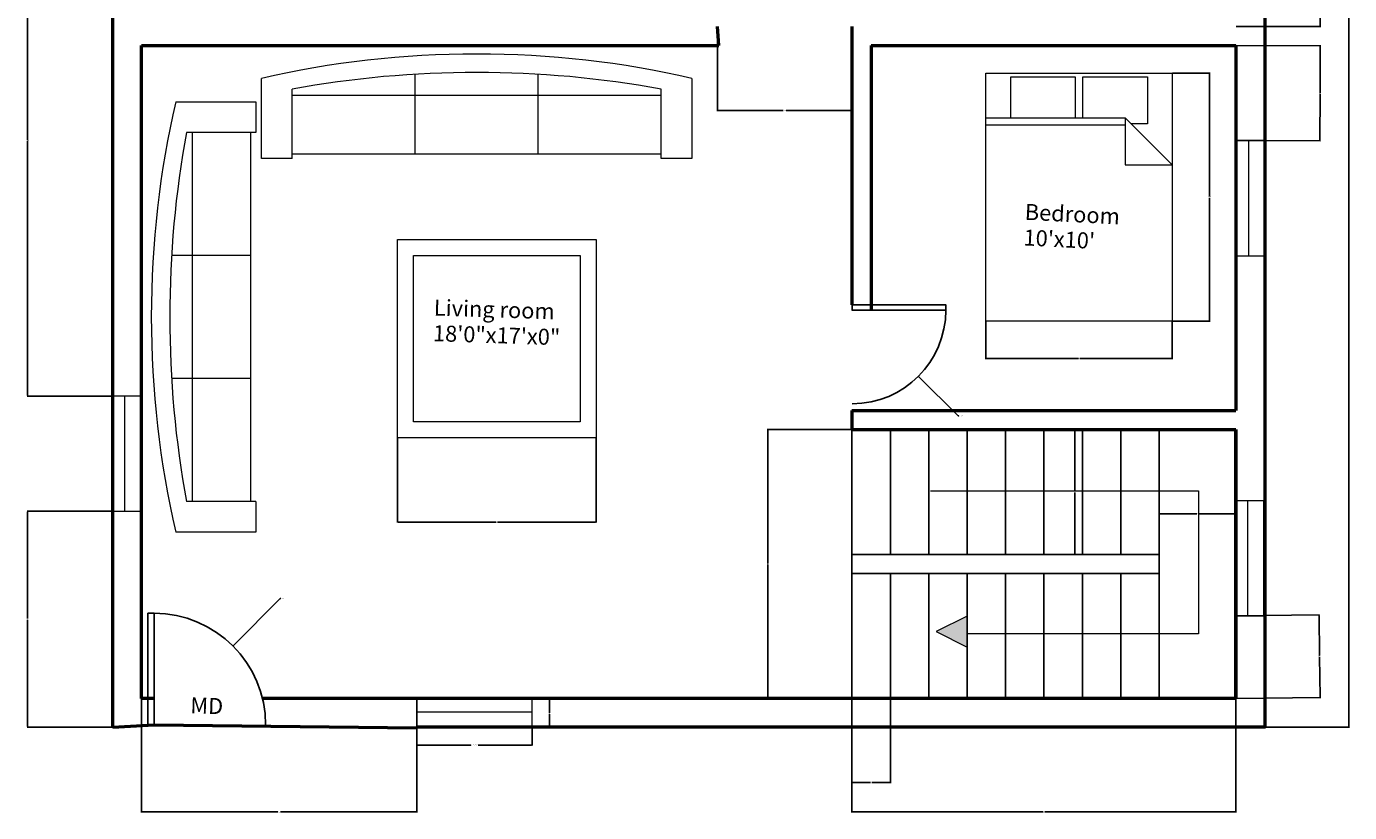
# Model space of a CAD drawing. Units: feet. Extents: x 2128 to 3163, y 1733 to 2266.
# Tile 2 of 3: x 2750 to 3163, y 1733 to 1979. Entities that reach past the tile are written whole.
import ezdxf

# ---------------------------------------------------------------- set-up
doc = ezdxf.new("R2010")
doc.units = ezdxf.units.FT
for name, color, linetype, lineweight in [('A-ANNO-DIMS', 2, 'Continuous', 18), ('A-ANNO-SYMB', 2, 'Continuous', 18), ('A-ANNO-TEXT', 7, 'Continuous', 18), ('A-AREA-IDEN', 7, 'Continuous', 18), ('A-DOOR', 3, 'Continuous', 25), ('A-FLOR-STRS', 7, 'Continuous', 25), ('A-FURN', 8, 'Continuous', 18), ('A-GLAZ', 4, 'Continuous', 18), ('A-WALL', 7, 'Continuous', 50)]:
    doc.layers.add(name, color=color, linetype=linetype, lineweight=lineweight)
doc.styles.get("Standard").update_dxf_attribs({"font": 'arial.ttf'})
doc.dimstyles.get("Standard").update_dxf_attribs({"dimtxt": 0.18, "dimasz": 0.18, "dimexe": 0.18, "dimexo": 0.0625, "dimgap": 0.09, "dimtad": 0, "dimtih": 1, "dimtoh": 1, "dimdec": 4, "dimzin": 0, "dimdsep": 46, "dimtxsty": 'Standard', "dimcen": 0.09, "dimadec": 0, "dimazin": 0, "dimtfac": 1, "dimtdec": 4, "dimtofl": 0, "dimtmove": 0, "dimatfit": 3, "dimfxl": 1, "dimtolj": 1, "dimtzin": 0, "dimarcsym": 0})

# ---------------------------------------------------------------- blocks, each defined once
blk = doc.blocks.new('Bed - Queen')
for p, q in [((0, -80.00003), (0, 0)), ((0, 0), (59.99999, 0)), ((59.99999, 0), (59.99999, -80.00003)), ((7.99999, -1.2), (28.79998, -1.2)), ((7.99999, -14.4), (7.99999, -1.2)), ((28.79998, -1.2), (28.79998, -14.4)), ((31.19999, -1.2), (51.99999, -1.2)), ((31.19999, -14.4), (31.19999, -1.2)), ((51.99999, -1.2), (51.99999, -16.4)), ((0, -14.4), (44.8, -14.4)), ((44.8, -16.8), (0, -16.8)), ((59.99999, -29.6), (44.8, -14.4)), ((44.8, -14.4), (44.8, -29.6)), ((51.99999, -16.4), (46.79936, -16.4)), ((44.8, -29.6), (59.99999, -29.6)), ((59.99999, -80.00003), (0, -80.00003))]:
    blk.add_line(p, q)
blk = doc.blocks.new('Sofa - Roundback 7 ft.')
for p, q in [((-12.00002, -32.4421), (-12.00003, -6.5971)), ((11.99997, -32.4421), (11.99998, -6.5971)), ((-36.000027, -34), (-36.000027, -11.4696)), ((35.99998, -34), (35.99998, -11.4696)), ((-35.999844, -13.3819), (35.9998, -13.3819)), ((-36.000027, -32.4421), (35.99998, -32.4421))]:
    blk.add_line(p, q)
for points in [[(-36.000027, -34), (-42.000027, -34), (-42.000027, -8)], [(41.99998, -8), (41.99998, -34), (35.99998, -34)]]:
    blk.add_lwpolyline(points)
for centre, radius, start, end in [((0, -114.25), 114.25, 68.43141, 111.5686), ((-0.00001, -127.1968), 121.1968, 72.72033, 107.2797)]:
    blk.add_arc(centre, radius, start, end)
blk = doc.blocks.new('DOOR-INTERIOR-SWING')
blk.add_lwpolyline([(1.63, 0), (0, 0), (0, 29.25), (1.63, 29.25)], close=True)
blk.add_arc((1.63, 0), 29.25, 0, 90)
blk = doc.blocks.new('WIN-SINGLE-36')
blk.add_line((0.01, 4.96), (35.9, 4.96))
blk.add_lwpolyline([(36, 9), (0, 9), (0, 0), (36, 0)], close=True)
blk = doc.blocks.new('*D9')
at = {"layer": 'A-ANNO-DIMS', "color": 0, "lineweight": -2, "transparency": 16777216}
for p, q in [((2871.76, 1759.28), (2871.76, 1753.77)), ((2907.76, 1759.28), (2907.76, 1753.77)), ((2871.94, 1753.95), (2888.65, 1753.95)), ((2907.58, 1753.95), (2890.88, 1753.95))]:
    blk.add_line(p, q, dxfattribs=at)
at = {"layer": 'A-ANNO-DIMS', "color": 0, "transparency": 16777216}
for points in [[(2871.94, 1753.98), (2871.94, 1753.92), (2871.76, 1753.95)], [(2907.58, 1753.98), (2907.58, 1753.92), (2907.76, 1753.95)]]:
    blk.add_solid(points, dxfattribs=at)
at = {"layer": 'Defpoints', "color": 0, "transparency": 16777216}
for p in [(2871.76, 1759.35), (2907.76, 1759.35), (2907.76, 1753.95)]:
    blk.add_point(p, dxfattribs=at)
at = {"layer": 'A-ANNO-DIMS', "color": 0, "transparency": 16777216, "insert": (2889.76, 1753.95), "char_height": 0.18, "attachment_point": 5}
blk.add_mtext('\\A1;WINDOW 36 TYP.', dxfattribs=at)
blk = doc.blocks.new('*D10')
at = {"layer": 'A-ANNO-DIMS', "color": 0, "lineweight": -2, "transparency": 16777216}
for p, q in [((2907.83, 1768.35), (2913.34, 1768.35)), ((2913.16, 1768.17), (2913.16, 1764.03)), ((2913.16, 1759.53), (2913.16, 1763.66)), ((2907.83, 1759.35), (2913.34, 1759.35))]:
    blk.add_line(p, q, dxfattribs=at)
at = {"layer": 'A-ANNO-DIMS', "color": 0, "transparency": 16777216}
for points in [[(2913.13, 1768.17), (2913.19, 1768.17), (2913.16, 1768.35)], [(2913.13, 1759.53), (2913.19, 1759.53), (2913.16, 1759.35)]]:
    blk.add_solid(points, dxfattribs=at)
at = {"layer": 'Defpoints', "color": 0, "transparency": 16777216}
for p in [(2907.76, 1768.35), (2913.16, 1768.35), (2907.76, 1759.35)]:
    blk.add_point(p, dxfattribs=at)
at = {"layer": 'A-ANNO-DIMS', "color": 0, "transparency": 16777216, "insert": (2913.16, 1763.85), "char_height": 0.18, "attachment_point": 5}
blk.add_mtext('\\A1;9 TYP.', dxfattribs=at)
blk = doc.blocks.new('*D17')
at = {"layer": 'A-ANNO-DIMS', "color": 0, "lineweight": -2, "transparency": 16777216}
for p, q in [((3107.89, 1963.99), (3119.64, 1963.99)), ((3119.46, 1963.81), (3119.46, 1925.39)), ((3119.46, 1886.61), (3119.46, 1925.03)), ((3107.89, 1886.43), (3119.64, 1886.43))]:
    blk.add_line(p, q, dxfattribs=at)
at = {"layer": 'A-ANNO-DIMS', "color": 0, "transparency": 16777216}
for points in [[(3119.43, 1963.81), (3119.49, 1963.81), (3119.46, 1963.99)], [(3119.43, 1886.61), (3119.49, 1886.61), (3119.46, 1886.43)]]:
    blk.add_solid(points, dxfattribs=at)
at = {"layer": 'Defpoints', "color": 0, "transparency": 16777216}
for p in [(3107.82, 1963.99), (3119.46, 1963.99), (3107.82, 1886.43)]:
    blk.add_point(p, dxfattribs=at)
at = {"layer": 'A-ANNO-DIMS', "color": 0, "transparency": 16777216, "insert": (3119.46, 1925.21), "char_height": 0.18, "attachment_point": 5}
blk.add_mtext('\\A1;BED 78', dxfattribs=at)
blk = doc.blocks.new('*D18')
at = {"layer": 'A-ANNO-DIMS', "color": 0, "lineweight": -2, "transparency": 16777216}
for p, q in [((3049.6, 1886.36), (3049.6, 1874.61)), ((3107.82, 1886.36), (3107.82, 1874.61)), ((3049.78, 1874.79), (3078.49, 1874.79)), ((3107.64, 1874.79), (3078.93, 1874.79))]:
    blk.add_line(p, q, dxfattribs=at)
at = {"layer": 'A-ANNO-DIMS', "color": 0, "transparency": 16777216}
for points in [[(3049.78, 1874.82), (3049.78, 1874.76), (3049.6, 1874.79)], [(3107.64, 1874.82), (3107.64, 1874.76), (3107.82, 1874.79)]]:
    blk.add_solid(points, dxfattribs=at)
at = {"layer": 'Defpoints', "color": 0, "transparency": 16777216}
for p in [(3049.6, 1886.43), (3107.82, 1886.43), (3107.82, 1874.79)]:
    blk.add_point(p, dxfattribs=at)
at = {"layer": 'A-ANNO-DIMS', "color": 0, "transparency": 16777216, "insert": (3078.71, 1874.79), "char_height": 0.18, "attachment_point": 5}
blk.add_mtext('\\A1;58', dxfattribs=at)
blk = doc.blocks.new('*D26')
at = {"layer": 'A-ANNO-DIMS', "color": 0, "lineweight": -2, "transparency": 16777216}
for p, q in [((3136.8, 2239.55), (3163.22, 2239.55)), ((3163.04, 2239.37), (3163.04, 1999.73)), ((3163.04, 1759.73), (3163.04, 1999.36)), ((3136.8, 1759.55), (3163.22, 1759.55))]:
    blk.add_line(p, q, dxfattribs=at)
at = {"layer": 'A-ANNO-DIMS', "color": 0, "transparency": 16777216}
for points in [[(3163.01, 2239.37), (3163.07, 2239.37), (3163.04, 2239.55)], [(3163.01, 1759.73), (3163.07, 1759.73), (3163.04, 1759.55)]]:
    blk.add_solid(points, dxfattribs=at)
at = {"layer": 'Defpoints', "color": 0, "transparency": 16777216}
for p in [(3136.74, 2239.55), (3136.74, 1759.55), (3163.04, 1759.55)]:
    blk.add_point(p, dxfattribs=at)
at = {"layer": 'A-ANNO-DIMS', "color": 0, "transparency": 16777216, "insert": (3163.04, 1999.55), "char_height": 0.18, "attachment_point": 5}
blk.add_mtext('\\A1;480', dxfattribs=at)
blk = doc.blocks.new('*D29')
at = {"layer": 'A-ANNO-DIMS', "color": 0, "lineweight": -2, "transparency": 16777216}
for p, q in [((2785.74, 1768.48), (2785.74, 1732.87)), ((2871.76, 1768.28), (2871.76, 1732.87)), ((2785.92, 1733.05), (2828.36, 1733.05)), ((2871.58, 1733.05), (2829.14, 1733.05))]:
    blk.add_line(p, q, dxfattribs=at)
at = {"layer": 'A-ANNO-DIMS', "color": 0, "transparency": 16777216}
for points in [[(2785.92, 1733.08), (2785.92, 1733.02), (2785.74, 1733.05)], [(2871.58, 1733.08), (2871.58, 1733.02), (2871.76, 1733.05)]]:
    blk.add_solid(points, dxfattribs=at)
at = {"layer": 'Defpoints', "color": 0, "transparency": 16777216}
for p in [(2785.74, 1768.55), (2871.76, 1768.35), (2871.76, 1733.05)]:
    blk.add_point(p, dxfattribs=at)
at = {"layer": 'A-ANNO-DIMS', "color": 0, "transparency": 16777216, "insert": (2828.75, 1733.05), "char_height": 0.18, "attachment_point": 5}
blk.add_mtext('\\A1;86.03', dxfattribs=at)
blk = doc.blocks.new('*D31')
at = {"layer": 'A-ANNO-DIMS', "color": 0, "lineweight": -2, "transparency": 16777216}
for p, q in [((3127.79, 2004.71), (3154.21, 2004.71)), ((3154.03, 2004.53), (3154.03, 1991.81)), ((3154.04, 1978.73), (3154.03, 1991.45)), ((3127.8, 1978.55), (3154.22, 1978.55))]:
    blk.add_line(p, q, dxfattribs=at)
at = {"layer": 'A-ANNO-DIMS', "color": 0, "transparency": 16777216}
for points in [[(3154.06, 2004.53), (3154, 2004.53), (3154.03, 2004.71)], [(3154.07, 1978.73), (3154.01, 1978.73), (3154.04, 1978.55)]]:
    blk.add_solid(points, dxfattribs=at)
at = {"layer": 'Defpoints', "color": 0, "transparency": 16777216}
for p in [(3127.73, 2004.71), (3127.74, 1978.55), (3154.04, 1978.55)]:
    blk.add_point(p, dxfattribs=at)
at = {"layer": 'A-ANNO-DIMS', "color": 0, "transparency": 16777216, "insert": (3154.03, 1991.63), "char_height": 0.18, "attachment_point": 5}
blk.add_mtext('\\A1;26.16', dxfattribs=at)
blk = doc.blocks.new('*D33')
at = {"layer": 'A-ANNO-DIMS', "color": 0, "lineweight": -2, "transparency": 16777216}
for p, q in [((3127.8, 1972.55), (3154.22, 1972.49)), ((3154.04, 1972.32), (3154.01, 1957.84)), ((3153.98, 1943), (3154.01, 1957.48)), ((3127.74, 1942.87), (3154.16, 1942.82))]:
    blk.add_line(p, q, dxfattribs=at)
at = {"layer": 'A-ANNO-DIMS', "color": 0, "transparency": 16777216}
for points in [[(3154.01, 1972.32), (3154.07, 1972.32), (3154.04, 1972.5)], [(3153.95, 1943), (3154.01, 1943), (3153.98, 1942.82)]]:
    blk.add_solid(points, dxfattribs=at)
at = {"layer": 'Defpoints', "color": 0, "transparency": 16777216}
for p in [(3127.74, 1972.55), (3127.68, 1942.87), (3153.98, 1942.82)]:
    blk.add_point(p, dxfattribs=at)
at = {"layer": 'A-ANNO-DIMS', "color": 0, "transparency": 16777216, "insert": (3154.01, 1957.66), "char_height": 0.18, "attachment_point": 5}
blk.add_mtext('\\A1;29.67', dxfattribs=at)
blk = doc.blocks.new('*D34')
at = {"layer": 'A-ANNO-DIMS', "color": 0, "lineweight": -2, "transparency": 16777216}
for p, q in [((3127.48, 1794.33), (3153.9, 1794.66)), ((3153.72, 1794.48), (3153.87, 1781.94)), ((3154.03, 1769.05), (3153.88, 1781.58)), ((3127.8, 1768.55), (3154.22, 1768.87))]:
    blk.add_line(p, q, dxfattribs=at)
at = {"layer": 'A-ANNO-DIMS', "color": 0, "transparency": 16777216}
for points in [[(3153.75, 1794.48), (3153.69, 1794.48), (3153.72, 1794.66)], [(3154.06, 1769.05), (3154, 1769.05), (3154.04, 1768.87)]]:
    blk.add_solid(points, dxfattribs=at)
at = {"layer": 'Defpoints', "color": 0, "transparency": 16777216}
for p in [(3127.42, 1794.33), (3127.74, 1768.55), (3154.04, 1768.87)]:
    blk.add_point(p, dxfattribs=at)
at = {"layer": 'A-ANNO-DIMS', "color": 0, "transparency": 16777216, "insert": (3153.88, 1781.76), "char_height": 0.18, "attachment_point": 5}
blk.add_mtext('\\A1;25.79', dxfattribs=at)
blk = doc.blocks.new('*D35')
at = {"layer": 'A-ANNO-DIMS', "color": 0, "lineweight": -2, "transparency": 16777216}
for p, q in [((3007.67, 1852.55), (2981.26, 1852.55)), ((2981.44, 1852.37), (2981.44, 1810.73)), ((2981.44, 1768.73), (2981.44, 1810.36)), ((3007.67, 1768.55), (2981.26, 1768.55))]:
    blk.add_line(p, q, dxfattribs=at)
at = {"layer": 'A-ANNO-DIMS', "color": 0, "transparency": 16777216}
for points in [[(2981.41, 1852.37), (2981.47, 1852.37), (2981.44, 1852.55)], [(2981.41, 1768.73), (2981.47, 1768.73), (2981.44, 1768.55)]]:
    blk.add_solid(points, dxfattribs=at)
at = {"layer": 'Defpoints', "color": 0, "transparency": 16777216}
for p in [(2981.44, 1852.55), (3007.74, 1852.55), (3007.74, 1768.55)]:
    blk.add_point(p, dxfattribs=at)
at = {"layer": 'A-ANNO-DIMS', "color": 0, "transparency": 16777216, "insert": (2981.44, 1810.55), "char_height": 0.18, "attachment_point": 5}
blk.add_mtext('\\A1;84', dxfattribs=at)
blk = doc.blocks.new('*D36')
at = {"layer": 'A-ANNO-DIMS', "color": 0, "lineweight": -2, "transparency": 16777216}
for p, q in [((3007.74, 1768.48), (3007.74, 1732.87)), ((3127.74, 1768.48), (3127.74, 1732.87)), ((3007.92, 1733.05), (3067.46, 1733.05)), ((3127.56, 1733.05), (3068.02, 1733.05))]:
    blk.add_line(p, q, dxfattribs=at)
at = {"layer": 'A-ANNO-DIMS', "color": 0, "transparency": 16777216}
for points in [[(3007.92, 1733.08), (3007.92, 1733.02), (3007.74, 1733.05)], [(3127.56, 1733.08), (3127.56, 1733.02), (3127.74, 1733.05)]]:
    blk.add_solid(points, dxfattribs=at)
at = {"layer": 'Defpoints', "color": 0, "transparency": 16777216}
for p in [(3007.74, 1768.55), (3127.74, 1768.55), (3127.74, 1733.05)]:
    blk.add_point(p, dxfattribs=at)
at = {"layer": 'A-ANNO-DIMS', "color": 0, "transparency": 16777216, "insert": (3067.74, 1733.05), "char_height": 0.18, "attachment_point": 5}
blk.add_mtext('\\A1;120', dxfattribs=at)
blk = doc.blocks.new('*D37')
at = {"layer": 'A-ANNO-DIMS', "color": 0, "lineweight": -2, "transparency": 16777216}
for p, q in [((3007.74, 1768.48), (3007.74, 1742.07)), ((3019.74, 1768.48), (3019.74, 1742.07)), ((3007.92, 1742.25), (3013.53, 1742.25)), ((3019.56, 1742.25), (3013.95, 1742.25))]:
    blk.add_line(p, q, dxfattribs=at)
at = {"layer": 'A-ANNO-DIMS', "color": 0, "transparency": 16777216}
for points in [[(3007.92, 1742.28), (3007.92, 1742.22), (3007.74, 1742.25)], [(3019.56, 1742.28), (3019.56, 1742.22), (3019.74, 1742.25)]]:
    blk.add_solid(points, dxfattribs=at)
at = {"layer": 'Defpoints', "color": 0, "transparency": 16777216}
for p in [(3007.74, 1768.55), (3019.74, 1768.55), (3007.74, 1742.25)]:
    blk.add_point(p, dxfattribs=at)
at = {"layer": 'A-ANNO-DIMS', "color": 0, "transparency": 16777216, "insert": (3013.74, 1742.25), "char_height": 0.18, "attachment_point": 5}
blk.add_mtext('\\A1;12', dxfattribs=at)
blk = doc.blocks.new('*D38')
at = {"layer": 'A-ANNO-DIMS', "color": 0, "lineweight": -2, "transparency": 16777216}
for p, q in [((3103.74, 1852.48), (3103.74, 1826.07)), ((3127.74, 1852.48), (3127.74, 1826.07)), ((3103.92, 1826.25), (3115.52, 1826.25)), ((3127.56, 1826.25), (3115.96, 1826.25))]:
    blk.add_line(p, q, dxfattribs=at)
at = {"layer": 'A-ANNO-DIMS', "color": 0, "transparency": 16777216}
for points in [[(3103.92, 1826.28), (3103.92, 1826.22), (3103.74, 1826.25)], [(3127.56, 1826.28), (3127.56, 1826.22), (3127.74, 1826.25)]]:
    blk.add_solid(points, dxfattribs=at)
at = {"layer": 'Defpoints', "color": 0, "transparency": 16777216}
for p in [(3103.74, 1852.55), (3127.74, 1852.55), (3103.74, 1826.25)]:
    blk.add_point(p, dxfattribs=at)
at = {"layer": 'A-ANNO-DIMS', "color": 0, "transparency": 16777216, "insert": (3115.74, 1826.25), "char_height": 0.18, "attachment_point": 5}
blk.add_mtext('\\A1;24', dxfattribs=at)
blk = doc.blocks.new('*D39')
at = {"layer": 'A-ANNO-DIMS', "color": 0, "lineweight": -2, "transparency": 16777216}
for p, q in [((3103.67, 1852.55), (3077.26, 1852.55)), ((3077.44, 1852.37), (3077.44, 1833.23)), ((3077.44, 1813.73), (3077.44, 1832.86)), ((3103.67, 1813.55), (3077.26, 1813.55))]:
    blk.add_line(p, q, dxfattribs=at)
at = {"layer": 'A-ANNO-DIMS', "color": 0, "transparency": 16777216}
for points in [[(3077.41, 1852.37), (3077.47, 1852.37), (3077.44, 1852.55)], [(3077.41, 1813.73), (3077.47, 1813.73), (3077.44, 1813.55)]]:
    blk.add_solid(points, dxfattribs=at)
at = {"layer": 'Defpoints', "color": 0, "transparency": 16777216}
for p in [(3077.44, 1852.55), (3103.74, 1852.55), (3103.74, 1813.55)]:
    blk.add_point(p, dxfattribs=at)
at = {"layer": 'A-ANNO-DIMS', "color": 0, "transparency": 16777216, "insert": (3077.44, 1833.05), "char_height": 0.18, "attachment_point": 5}
blk.add_mtext('\\A1;39', dxfattribs=at)
blk = doc.blocks.new('*D40')
at = {"layer": 'A-ANNO-DIMS', "color": 0, "lineweight": -2, "transparency": 16777216}
for p, q in [((2776.42, 1827.05), (2749.94, 1827.05)), ((2750.12, 1826.87), (2750.12, 1793.48)), ((2750.12, 1759.73), (2750.12, 1793.11)), ((2776.67, 1759.55), (2749.94, 1759.55))]:
    blk.add_line(p, q, dxfattribs=at)
at = {"layer": 'A-ANNO-DIMS', "color": 0, "transparency": 16777216}
for points in [[(2750.09, 1826.87), (2750.15, 1826.87), (2750.12, 1827.05)], [(2750.09, 1759.73), (2750.15, 1759.73), (2750.12, 1759.55)]]:
    blk.add_solid(points, dxfattribs=at)
at = {"layer": 'Defpoints', "color": 0, "transparency": 16777216}
for p in [(2750.12, 1827.05), (2776.49, 1827.05), (2776.74, 1759.55)]:
    blk.add_point(p, dxfattribs=at)
at = {"layer": 'A-ANNO-DIMS', "color": 0, "transparency": 16777216, "insert": (2750.12, 1793.3), "char_height": 0.18, "attachment_point": 5}
blk.add_mtext('\\A1;67.5', dxfattribs=at)
blk = doc.blocks.new('*D41')
at = {"layer": 'A-ANNO-DIMS', "color": 0, "lineweight": -2, "transparency": 16777216}
for p, q in [((2776.5, 2022.82), (2749.94, 2022.82)), ((2750.12, 2022.64), (2750.12, 1943.11)), ((2750.12, 1863.23), (2750.12, 1942.75)), ((2776.42, 1863.05), (2749.94, 1863.05))]:
    blk.add_line(p, q, dxfattribs=at)
at = {"layer": 'A-ANNO-DIMS', "color": 0, "transparency": 16777216}
for points in [[(2750.09, 2022.64), (2750.15, 2022.64), (2750.12, 2022.82)], [(2750.09, 1863.23), (2750.15, 1863.23), (2750.12, 1863.05)]]:
    blk.add_solid(points, dxfattribs=at)
at = {"layer": 'Defpoints', "color": 0, "transparency": 16777216}
for p in [(2750.12, 2022.82), (2776.56, 2022.82), (2776.49, 1863.05)]:
    blk.add_point(p, dxfattribs=at)
at = {"layer": 'A-ANNO-DIMS', "color": 0, "transparency": 16777216, "insert": (2750.12, 1942.93), "char_height": 0.18, "attachment_point": 5}
blk.add_mtext('\\A1;159.77', dxfattribs=at)
blk = doc.blocks.new('*D45')
at = {"layer": 'A-ANNO-DIMS', "color": 0, "lineweight": -2, "transparency": 16777216}
for p, q in [((2865.75, 1849.89), (2865.75, 1823.47)), ((2927.75, 1849.89), (2927.75, 1823.47)), ((2865.93, 1823.65), (2896.53, 1823.65)), ((2927.57, 1823.65), (2896.97, 1823.65))]:
    blk.add_line(p, q, dxfattribs=at)
at = {"layer": 'A-ANNO-DIMS', "color": 0, "transparency": 16777216}
for points in [[(2865.93, 1823.68), (2865.93, 1823.62), (2865.75, 1823.65)], [(2927.57, 1823.68), (2927.57, 1823.62), (2927.75, 1823.65)]]:
    blk.add_solid(points, dxfattribs=at)
at = {"layer": 'Defpoints', "color": 0, "transparency": 16777216}
for p in [(2865.75, 1849.95), (2927.75, 1849.95), (2865.75, 1823.65)]:
    blk.add_point(p, dxfattribs=at)
at = {"layer": 'A-ANNO-DIMS', "color": 0, "transparency": 16777216, "insert": (2896.75, 1823.65), "char_height": 0.18, "attachment_point": 5}
blk.add_mtext('\\A1;62', dxfattribs=at)
blk = doc.blocks.new('*D49')
at = {"layer": 'A-ANNO-DIMS', "color": 0, "lineweight": -2, "transparency": 16777216}
for p, q in [((2965.74, 1978.48), (2965.74, 1952.07)), ((3007.74, 1978.48), (3007.74, 1952.07)), ((2965.92, 1952.25), (2986.27, 1952.25)), ((3007.56, 1952.25), (2987.21, 1952.25))]:
    blk.add_line(p, q, dxfattribs=at)
at = {"layer": 'A-ANNO-DIMS', "color": 0, "transparency": 16777216}
for points in [[(2965.92, 1952.28), (2965.92, 1952.22), (2965.74, 1952.25)], [(3007.56, 1952.28), (3007.56, 1952.22), (3007.74, 1952.25)]]:
    blk.add_solid(points, dxfattribs=at)
at = {"layer": 'Defpoints', "color": 0, "transparency": 16777216}
for p in [(2965.74, 1978.55), (3007.74, 1978.55), (2965.74, 1952.25)]:
    blk.add_point(p, dxfattribs=at)
at = {"layer": 'A-ANNO-DIMS', "color": 0, "transparency": 16777216, "insert": (2986.74, 1952.25), "char_height": 0.18, "attachment_point": 5}
blk.add_mtext('\\A1;41.996', dxfattribs=at)
blk = doc.blocks.new('*D52')
at = {"layer": 'A-ANNO-DIMS', "color": 0, "lineweight": -2, "transparency": 16777216}
for p, q in [((2829.07, 1799.71), (2814.41, 1785.05)), ((2829.25, 1799.71), (2829.07, 1799.71)), ((2789.55, 1760.28), (2789.73, 1760.28)), ((2789.64, 1760.19), (2789.64, 1760.37))]:
    blk.add_line(p, q, dxfattribs=at)
at = {"layer": 'A-ANNO-DIMS', "color": 0, "transparency": 16777216}
blk.add_solid([(2814.39, 1785.08), (2814.43, 1785.03), (2814.28, 1784.93)], dxfattribs=at)
at = {"layer": 'Defpoints', "color": 0, "transparency": 16777216}
for p in [(2814.28, 1784.93), (2789.64, 1760.28)]:
    blk.add_point(p, dxfattribs=at)
at = {"layer": 'A-ANNO-DIMS', "color": 0, "transparency": 16777216, "insert": (2829.8, 1799.71), "char_height": 0.18, "attachment_point": 5}
blk.add_mtext('\\A1;R34.854', dxfattribs=at)
blk = doc.blocks.new('*D53')
at = {"layer": 'A-ANNO-DIMS', "color": 0, "lineweight": -2, "transparency": 16777216}
for p, q in [((3007.75, 1889.9), (3007.93, 1889.9)), ((3007.84, 1889.81), (3007.84, 1889.99)), ((3040.93, 1856.8), (3028.65, 1869.08)), ((3041.11, 1856.8), (3040.93, 1856.8))]:
    blk.add_line(p, q, dxfattribs=at)
at = {"layer": 'A-ANNO-DIMS', "color": 0, "transparency": 16777216}
blk.add_solid([(3028.67, 1869.11), (3028.63, 1869.06), (3028.52, 1869.21)], dxfattribs=at)
at = {"layer": 'Defpoints', "color": 0, "transparency": 16777216}
for p in [(3007.84, 1889.9), (3028.52, 1869.21)]:
    blk.add_point(p, dxfattribs=at)
at = {"layer": 'A-ANNO-DIMS', "color": 0, "transparency": 16777216, "insert": (3041.86, 1856.8), "char_height": 0.18, "attachment_point": 5}
blk.add_mtext('\\A1;3X R29.255', dxfattribs=at)

msp = doc.modelspace()

# ---------------------------------------------------------------- hatches: boundary and pattern name
at = {"layer": 'A-ANNO-SYMB'}
h = msp.add_hatch(color=256, dxfattribs=at)
h.dxf.hatch_style = 1
h.paths.add_polyline_path([(3043.737, 1794.2137), (3034.0015, 1789.4301), (3043.737, 1784.5668)])

# ---------------------------------------------------------------- linework, layer by layer
for p, q in [((3032.3072, 1833.4364), (3116.0327, 1833.4364)), ((3116.0327, 1833.4364), (3116.0327, 1788.7203)), ((3043.737, 1794.2137), (3034.0015, 1789.4301)), ((3034.0015, 1789.4301), (3043.7249, 1784.5728)), ((3116.0327, 1788.7203), (3043.8822, 1788.7203))]:
    msp.add_line(p, q, dxfattribs=at)
at = {"layer": 'A-DOOR'}
msp.add_lwpolyline([(2789.6368, 1760.281), (2787.7005, 1760.281), (2787.7005, 1795.1352), (2789.6368, 1795.1352)], close=True, dxfattribs=at)
msp.add_arc((2789.6368, 1760.281), 34.8542, 0, 90, dxfattribs=at)
at = {"layer": 'A-FLOR-STRS'}
for p, q in [((3007.737, 1768.546), (3007.737, 1852.546)), ((3019.737, 1813.546), (3019.737, 1852.546)), ((3031.737, 1813.546), (3031.737, 1852.546)), ((3043.737, 1813.546), (3043.737, 1852.546)), ((3055.737, 1813.546), (3055.737, 1852.546)), ((3067.737, 1813.546), (3067.737, 1852.546)), ((3079.737, 1813.546), (3079.737, 1852.546)), ((3091.737, 1813.546), (3091.737, 1852.546)), ((3103.737, 1768.546), (3103.737, 1852.546)), ((3007.737, 1813.546), (3103.737, 1813.546)), ((3007.737, 1807.546), (3103.737, 1807.546)), ((3019.737, 1768.546), (3019.737, 1807.546)), ((3031.737, 1768.546), (3031.737, 1807.546)), ((3043.737, 1768.546), (3043.737, 1807.546)), ((3055.737, 1768.546), (3055.737, 1807.546)), ((3067.737, 1768.546), (3067.737, 1807.546)), ((3079.737, 1768.546), (3079.737, 1807.546)), ((3091.737, 1768.546), (3091.737, 1807.546))]:
    msp.add_line(p, q, dxfattribs=at)
at = {"layer": 'A-FURN'}
for points in [[(2865.7512, 1911.9544), (2927.7512, 1911.9544), (2927.7512, 1849.9544), (2865.7512, 1849.9544)], [(2870.7512, 1906.9544), (2922.7512, 1906.9544), (2922.7512, 1854.9544), (2870.7512, 1854.9544)]]:
    msp.add_lwpolyline(points, close=True, dxfattribs=at)
at = {"layer": 'A-WALL'}
for p, q in [((2966.0879, 1972.546), (2965.7414, 1978.546)), ((3007.737, 1978.546), (3007.737, 1891.5229)), ((2785.737, 1768.546), (2785.737, 1972.546)), ((2785.737, 1972.546), (2953.737, 1972.546)), ((2953.737, 1972.546), (2966.0879, 1972.546)), ((3013.737, 1972.546), (3013.737, 1889.8976)), ((3013.737, 1972.546), (3127.737, 1972.546)), ((3127.737, 1972.546), (3127.737, 1858.546)), ((3007.8364, 1891.5229), (3007.737, 1891.5229)), ((3007.737, 1858.546), (3127.737, 1858.546)), ((3007.737, 1858.546), (3007.737, 1852.546)), ((3007.737, 1852.546), (3127.737, 1852.546)), ((3127.737, 1768.546), (3127.737, 1852.546)), ((3127.737, 1852.546), (3127.737, 1768.546)), ((2789.6368, 1768.546), (2785.737, 1768.546)), ((3127.737, 1768.546), (2823.4969, 1768.546)), ((2776.737, 1759.546), (2789.6368, 1760.281)), ((2789.6368, 1760.281), (2871.7638, 1759.3457))]:
    msp.add_line(p, q, dxfattribs=at)
msp.add_lwpolyline([(2776.737, 1759.546), (2776.737, 2239.546), (3136.737, 2239.546), (3136.737, 1759.546), (2871.7638, 1759.546)], dxfattribs=at)

# ---------------------------------------------------------------- block references
at = {"layer": 'A-DOOR', "rotation": 270.0000000000013}
msp.add_blockref('DOOR-INTERIOR-SWING', (3007.8364, 1891.5232), dxfattribs=at)
at = {"layer": 'A-FURN', "xscale": 1.601553536944322, "yscale": 0.9600654288777931, "zscale": 1.601553536944322}
msp.add_blockref('Sofa - Roundback 7 ft.', (2890.4559, 1969.9316), dxfattribs=at)
at = {"layer": 'A-FURN'}
for name, p, xscale, yscale, zscale, rotation in [('Bed - Queen', (3049.5954, 1963.9936), -0.9704664129428286, -0.9695930824229791, 0.9704664129428286, 180), ('Sofa - Roundback 7 ft.', (2788.7678, 1887.7649), 1.601553536944322, 0.9600654288777931, 1.601553536944322, 90)]:
    msp.add_blockref(name, p, dxfattribs=dict(at, xscale=xscale, yscale=yscale, zscale=zscale, rotation=rotation))
at = {"layer": 'A-GLAZ'}
for p, rotation in [((3136.6792, 1906.8748), 89.99999999999808), ((2785.487, 1827.0466), 90.0000000000003), ((3136.4194, 1794.3335), 89.99999999999523)]:
    msp.add_blockref('WIN-SINGLE-36', p, dxfattribs=dict(at, rotation=rotation))
msp.add_blockref('WIN-SINGLE-36', (2871.7641, 1759.3461), dxfattribs=at)

# ---------------------------------------------------------------- texts
at = {"layer": 'A-ANNO-TEXT'}
msp.add_text('MD', height=5, rotation=358.123817, dxfattribs=at).set_placement((2800.9111, 1763.9148))
at = {"layer": 'A-AREA-IDEN'}
for s, rotation, p in [('Bedroom', 357.140175, (3061.6536, 1918.1507)), ("10'x10'", 357.140175, (3061.2529, 1910.1286)), ('Living room', 358.123817, (2876.9926, 1888.2293)), ('18\'0"x17\'x0"', 358.123817, (2876.7297, 1880.2015))]:
    msp.add_text(s, height=5, rotation=rotation, dxfattribs=at).set_placement(p)

# ---------------------------------------------------------------- dimensions: what is measured, and where the dimension line sits
at = {"layer": 'A-ANNO-DIMS'}
for base, p1, p2, angle, override, picture, middle in [((3163.037, 1759.546), (3136.737, 2239.546), (3136.737, 1759.546), 90, {"dimdec": 0, "dimlfac": 1, "dimrnd": 0, "dimzin": 0, "dimdsep": 46, "dimlunit": 2}, '*D26', (3163.037, 1999.546)), ((2750.1232, 2022.8164), (2776.4874, 1863.0464), (2776.5598, 2022.8164), 90, {"dimdec": 2, "dimlfac": 1, "dimrnd": 0, "dimzin": 0, "dimdsep": 46, "dimlunit": 2}, '*D41', (2750.1232, 1942.9314)), ((3154.037, 1978.5514), (3127.7317, 2004.7069), (3127.737, 1978.546), 270.011744, {"dimdec": 2, "dimlfac": 1, "dimrnd": 0, "dimzin": 0, "dimdsep": 46, "dimlunit": 2}, '*D31', (3154.0343, 1991.6318)), ((2965.7414, 1952.246), (3007.737, 1978.546), (2965.7414, 1978.546), 180, {"dimdec": 3, "dimlfac": 1, "dimrnd": 0, "dimzin": 0, "dimdsep": 46, "dimlunit": 2}, '*D49', (2986.7392, 1952.246)), ((3153.9796, 1942.8237), (3127.737, 1972.546), (3127.6796, 1942.8745), 269.889221, {"dimdec": 2, "dimlfac": 1, "dimrnd": 0, "dimzin": 0, "dimdsep": 46, "dimlunit": 2}, '*D33', (3154.0083, 1957.6594)), ((2981.437, 1852.546), (3007.737, 1768.546), (3007.737, 1852.546), 90, {"dimdec": 0, "dimlfac": 1, "dimrnd": 0, "dimzin": 0, "dimdsep": 46, "dimlunit": 2}, '*D35', (2981.437, 1810.546)), ((3077.437, 1852.546), (3103.737, 1813.546), (3103.737, 1852.546), 90, {"dimdec": 0, "dimlfac": 1, "dimrnd": 0, "dimzin": 0, "dimdsep": 46, "dimlunit": 2}, '*D39', (3077.437, 1833.046)), ((3103.737, 1826.246), (3127.737, 1852.546), (3103.737, 1852.546), 180, {"dimdec": 0, "dimlfac": 1, "dimrnd": 0, "dimzin": 0, "dimdsep": 46, "dimlunit": 2}, '*D38', (3115.737, 1826.246)), ((2865.7512, 1823.6544), (2927.7512, 1849.9544), (2865.7512, 1849.9544), 180, {"dimdec": 0, "dimlfac": 1, "dimrnd": 0, "dimzin": 0, "dimdsep": 46, "dimlunit": 2}, '*D45', (2896.7512, 1823.6544)), ((2750.1232, 1827.0464), (2776.737, 1759.546), (2776.4874, 1827.0464), 90, {"dimdec": 1, "dimlfac": 1, "dimrnd": 0, "dimzin": 0, "dimdsep": 46, "dimlunit": 2}, '*D40', (2750.1232, 1793.2962)), ((3154.035, 1768.8694), (3127.4198, 1794.3332), (3127.737, 1768.546), 270.704729, {"dimdec": 2, "dimlfac": 1, "dimrnd": 0, "dimzin": 0, "dimdsep": 46, "dimlunit": 2}, '*D34', (3153.8764, 1781.7631)), ((3007.737, 1742.246), (3019.737, 1768.546), (3007.737, 1768.546), 180, {"dimdec": 0, "dimlfac": 1, "dimrnd": 0, "dimzin": 0, "dimdsep": 46, "dimlunit": 2}, '*D37', (3013.737, 1742.246))]:
    dim = msp.add_linear_dim(base=base, p1=p1, p2=p2, angle=angle, dimstyle='Standard', override=override, dxfattribs=at)
    dim.commit()
    dim.dimension.update_dxf_attribs({"geometry": picture, "text_midpoint": middle})
for base, p1, p2, text, picture, middle in [((3119.4585, 1963.9936), (3107.8234, 1886.4261), (3107.8234, 1963.9936), 'BED <>', '*D17', (3119.4585, 1925.2099)), ((2913.1638, 1768.3457), (2907.7638, 1759.3457), (2907.7638, 1768.3457), '<> TYP.', '*D10', (2913.1638, 1763.8457))]:
    dim = msp.add_linear_dim(base=base, p1=p1, p2=p2, angle=90, text=text, dimstyle='Standard', override={"dimdec": 0, "dimlfac": 1, "dimrnd": 0, "dimzin": 0, "dimdsep": 46, "dimlunit": 2}, dxfattribs=at)
    dim.commit()
    dim.dimension.update_dxf_attribs({"geometry": picture, "text_midpoint": middle})
dim = msp.add_radius_dim(center=(3007.8364, 1889.8976), mpoint=(3028.5226, 1869.2114), text='3X <>', dimstyle='Standard', override={"dimdec": 3, "dimlfac": 1, "dimrnd": 0, "dimzin": 0, "dimdsep": 46, "dimlunit": 2}, dxfattribs=at)
dim.commit()
dim.dimension.update_dxf_attribs({"geometry": '*D53', "text_midpoint": (3041.8581, 1856.7996), "dimtype": 164})
for base, p1, p2, override, picture, middle in [((3107.8234, 1874.791), (3049.5954, 1886.4261), (3107.8234, 1886.4261), {"dimdec": 0, "dimlfac": 1, "dimrnd": 0, "dimzin": 0, "dimdsep": 46, "dimlunit": 2}, '*D18', (3078.7094, 1874.791)), ((2871.7638, 1733.0457), (2785.737, 1768.546), (2871.7638, 1768.3457), {"dimdec": 2, "dimlfac": 1, "dimrnd": 0, "dimzin": 0, "dimdsep": 46, "dimlunit": 2}, '*D29', (2828.7504, 1733.0457)), ((3127.737, 1733.0457), (3007.737, 1768.546), (3127.737, 1768.546), {"dimdec": 0, "dimlfac": 1, "dimrnd": 0, "dimzin": 0, "dimdsep": 46, "dimlunit": 2}, '*D36', (3067.737, 1733.0457))]:
    dim = msp.add_linear_dim(base=base, p1=p1, p2=p2, dimstyle='Standard', override=override, dxfattribs=at)
    dim.commit()
    dim.dimension.update_dxf_attribs({"geometry": picture, "text_midpoint": middle})
dim = msp.add_radius_dim(center=(2789.6368, 1760.281), mpoint=(2814.282, 1784.927), dimstyle='Standard', override={"dimdec": 3, "dimlfac": 1, "dimrnd": 0, "dimzin": 0, "dimdsep": 46, "dimlunit": 2}, dxfattribs=at)
dim.commit()
dim.dimension.update_dxf_attribs({"geometry": '*D52', "text_midpoint": (2829.7985, 1799.7147), "dimtype": 164})
dim = msp.add_linear_dim(base=(2907.7638, 1753.9457), p1=(2871.7638, 1759.3457), p2=(2907.7638, 1759.3457), text='WINDOW <> TYP.', dimstyle='Standard', override={"dimdec": 0, "dimlfac": 1, "dimrnd": 0, "dimzin": 0, "dimdsep": 46, "dimlunit": 2}, dxfattribs=at)
dim.commit()
dim.dimension.update_dxf_attribs({"geometry": '*D9', "text_midpoint": (2889.7638, 1753.9457)})

doc.saveas('drawing.dxf')
